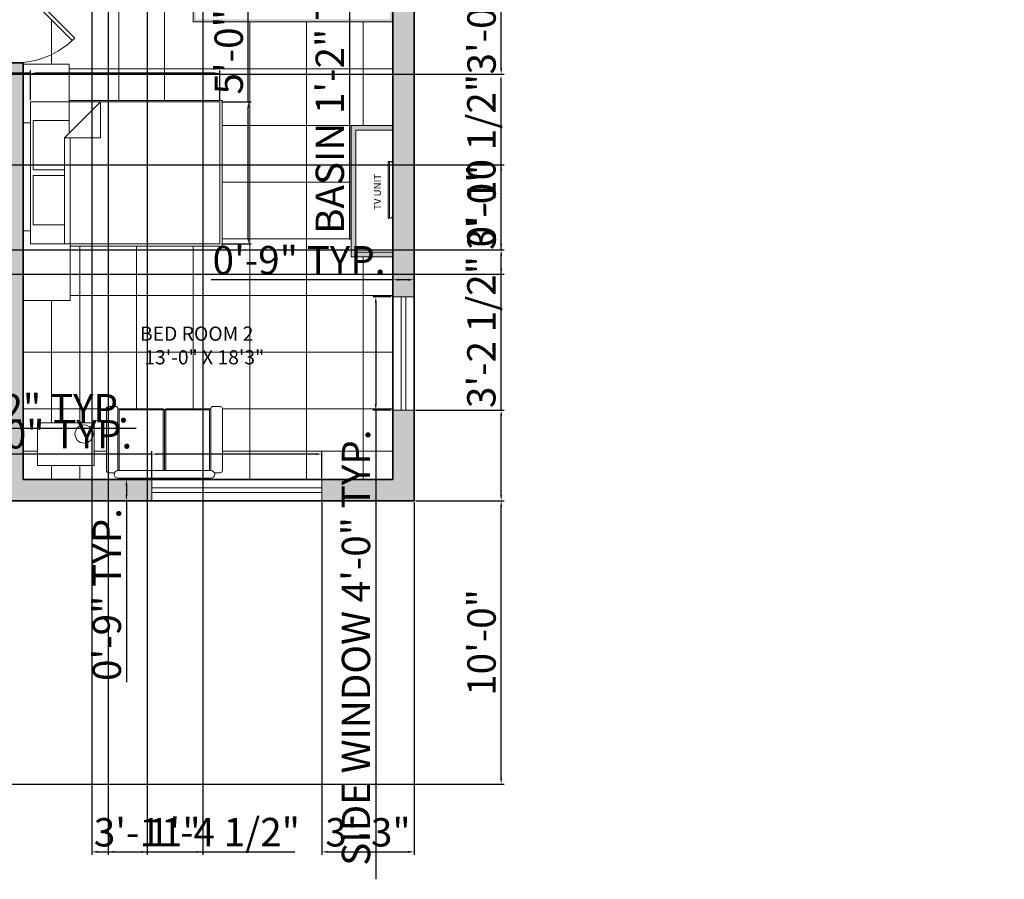
# Model space of a CAD drawing. Units: millimetres. Extents: x 542930 to 543750, y 628093 to 628738.
# Tile 8 of 14: x 543333 to 543750, y 628093 to 628458. Entities that reach past the tile are written whole.
import ezdxf

# ---------------------------------------------------------------- set-up
doc = ezdxf.new("R2010")
doc.units = ezdxf.units.MM
for name, color, linetype, lineweight in [('A-ANNO-DIMS', 2, 'Continuous', 18), ('A-EQPM', 9, 'Continuous', 18), ('A-EQPM-PATT', 9, 'Continuous', 13), ('A-FURN', 8, 'Continuous', 18), ('A-FURN-MILL', 8, 'Continuous', 18), ('A-FURN-PATT', 9, 'Continuous', 13), ('A-WALL', 7, 'Continuous', 35), ('DOORS', 30, 'Continuous', 18), ('WINDOW', 70, 'Continuous', 18)]:
    doc.layers.add(name, color=color, linetype=linetype, lineweight=lineweight)
for name, color, linetype, lineweight, true_color in [('A-ANNO-TEXT', 40, 'Continuous', 18, 0xf8d731), ('A-AREA-IDEN', 40, 'Continuous', 18, 0xf8d731), ('A-FLOR-PATT', 241, 'Continuous', 13, 0xf7abae), ('A-WALL-PATT', 251, 'Continuous', 13, 0x636466)]:
    doc.layers.add(name, color=color, linetype=linetype, lineweight=lineweight, true_color=true_color)
doc.styles.get("Standard").update_dxf_attribs({"font": 'arial.ttf'})
doc.dimstyles.new('ISO-25', dxfattribs={"dimtxt": 12, "dimasz": 2.5, "dimexe": 1.25, "dimexo": 0.625, "dimtad": 1, "dimdec": 0, "dimlunit": 3, "dimtxsty": 'Standard', "dimcen": 2.5, "dimadec": 0, "dimazin": 0, "dimtfac": 1, "dimtdec": 0, "dimtmove": 0, "dimatfit": 3, "dimfxl": 1, "dimarcsym": 0})

# ---------------------------------------------------------------- blocks, each defined once
blk = doc.blocks.new('*U2')
for p, q in [((0, 0), (0, -6)), ((40, 0), (40, -6))]:
    blk.add_line(p, q)
blk.add_lwpolyline([(0, 0), (28.28, 28.28), (29.52, 27.05), (1.24, -1.24)], close=True)
blk.add_arc((0, 0), 40, 0, 45)
blk = doc.blocks.new('Bed - Queen')
for p, q in [((0, -80.00003), (0, 0)), ((0, 0), (59.99999, 0)), ((59.99999, 0), (59.99999, -80.00003)), ((7.99999, -1.2), (28.79998, -1.2)), ((7.99999, -14.4), (7.99999, -1.2)), ((28.79998, -1.2), (28.79998, -14.4)), ((31.19999, -1.2), (51.99999, -1.2)), ((31.19999, -14.4), (31.19999, -1.2)), ((51.99999, -1.2), (51.99999, -16.4)), ((0, -14.4), (44.8, -14.4)), ((59.99999, -29.6), (44.8, -14.4)), ((44.8, -14.4), (44.8, -29.6)), ((51.99999, -16.4), (46.79936, -16.4)), ((44.8, -16.8), (0, -16.8)), ((44.8, -29.6), (59.99999, -29.6)), ((59.99999, -80.00003), (0, -80.00003))]:
    blk.add_line(p, q)
blk = doc.blocks.new('sofa')
for p, q in [((543001.62, 628230.38), (543001.62, 628182.38)), ((543010.62, 628230.38), (543045.62, 628230.38)), ((543091.62, 628230.38), (543091.62, 628182.38)), ((543045.62, 628229.38), (543045.62, 628182.38)), ((543046.62, 628228.78), (543046.62, 628182.38)), ((543010.62, 628176.38), (543082.62, 628176.38))]:
    blk.add_line(p, q)
for points in [[(543009.53, 628232.06), (543003.46, 628232.06, 0.414214), (543001.62, 628230.23)], [(543045.62, 628230.38, 0.623864), (543047.62, 628230.38), (543082.62, 628230.38), (543082.62, 628182.38), (543010.62, 628182.38), (543010.62, 628230.38, 0.297291), (543009.53, 628232.06)], [(543083.72, 628232.06, 0.297291), (543082.62, 628230.38), (543082.62, 628182.38)], [(543091.62, 628230.23, 0.414214), (543089.79, 628232.06), (543083.72, 628232.06)], [(543001.62, 628182.54, 0.414214), (543003.46, 628180.7), (543007.93, 628180.7)], [(543082.62, 628182.38, -1), (543082.62, 628176.38), (543082.62, 628175.38), (543010.62, 628175.38), (543010.62, 628176.38, -1), (543010.62, 628182.38)], [(543085.32, 628180.7), (543089.79, 628180.7, 0.414214), (543091.62, 628182.54)]]:
    blk.add_lwpolyline(points, format="xyb")
for points in [[(543011.62, 628182.38), (543011.62, 628229.38), (543045.62, 628229.38), (543045.62, 628229.4)], [(543047.62, 628182.38), (543047.62, 628229.38), (543047.62, 628229.4)], [(543047.62, 628229.38), (543081.62, 628229.38), (543081.62, 628182.38)]]:
    blk.add_lwpolyline(points)
blk.add_arc((543046.62, 628229.89), 1.11, 206.0829, 333.9171)
blk = doc.blocks.new('BEDROOM-END-TABLE')
for p, q in [((0, 0), (0, 18)), ((24.02, 18), (0, 18)), ((24.02, 0), (24.02, 18)), ((24.02, 0), (0, 0))]:
    blk.add_line(p, q)
blk.add_circle((19.74, 13.28), 3.85)
blk = doc.blocks.new('WIN-BEDROOM-FRONT')
for p, q in [((0, 9), (0, 0)), ((72, 9), (72, 0)), ((0, 5.5), (72, 5.5)), ((0, 3.5), (72, 3.5))]:
    blk.add_line(p, q)
blk = doc.blocks.new('WIN-BEDROOM-SIDE')
for p, q in [((0, 48), (9, 48)), ((3.5, 48), (3.5, 0)), ((5.5, 48), (5.5, 0)), ((0, 0), (9, 0))]:
    blk.add_line(p, q)
blk = doc.blocks.new('BED-SIDE-STAND')
for p, q in [((19.46, 24), (0, 24)), ((19.46, 0), (19.46, 24))]:
    blk.add_line(p, q)
blk = doc.blocks.new('*D35')
at = {"layer": 'A-ANNO-DIMS', "color": 0, "lineweight": -2, "transparency": 16777216}
for p, q in [((543473.87, 628509.97), (543471.13, 628509.97)), ((543472.38, 628507.47), (543472.38, 628498.35)), ((543473.87, 628495.85), (543471.13, 628495.85)), ((543472.38, 628495.85), (543472.38, 628364.52))]:
    blk.add_line(p, q, dxfattribs=at)
at = {"layer": 'A-ANNO-DIMS', "color": 0, "transparency": 16777216}
for points in [[(543471.96, 628507.47), (543472.79, 628507.47), (543472.38, 628509.97)], [(543471.96, 628498.35), (543472.79, 628498.35), (543472.38, 628495.85)]]:
    blk.add_solid(points, dxfattribs=at)
at = {"layer": 'Defpoints', "color": 0, "transparency": 16777216}
for p in [(543474.49, 628509.97), (543472.38, 628495.85), (543474.49, 628495.85)]:
    blk.add_point(p, dxfattribs=at)
at = {"layer": 'A-ANNO-DIMS', "color": 0, "transparency": 16777216, "insert": (543465.55, 628428.93), "char_height": 12, "attachment_point": 5, "rotation": 90}
blk.add_mtext('BASIN 1\'-2" TYP.', dxfattribs=at)
blk = doc.blocks.new('*D37')
at = {"layer": 'A-ANNO-DIMS', "color": 0, "lineweight": -2, "transparency": 16777216}
for p, q in [((543337.17, 628434.96), (543128.93, 628434.96)), ((543337.17, 628423.55), (543337.17, 628436.21)), ((543414.94, 628434.96), (543339.67, 628434.96)), ((543417.44, 628423.55), (543417.44, 628436.21))]:
    blk.add_line(p, q, dxfattribs=at)
at = {"layer": 'A-ANNO-DIMS', "color": 0, "transparency": 16777216}
for points in [[(543339.67, 628435.38), (543339.67, 628434.55), (543337.17, 628434.96)], [(543414.94, 628435.38), (543414.94, 628434.55), (543417.44, 628434.96)]]:
    blk.add_solid(points, dxfattribs=at)
at = {"layer": 'Defpoints', "color": 0, "transparency": 16777216}
for p in [(543337.17, 628434.96), (543337.17, 628422.92), (543417.44, 628422.92)]:
    blk.add_point(p, dxfattribs=at)
at = {"layer": 'A-ANNO-DIMS', "color": 0, "transparency": 16777216, "insert": (543231.8, 628442.16), "char_height": 12, "attachment_point": 5}
blk.add_mtext('QUEEN BED 6\'-8 1/2" TYP.', dxfattribs=at)
blk = doc.blocks.new('*D38')
at = {"layer": 'A-ANNO-DIMS', "color": 0, "lineweight": -2, "transparency": 16777216}
for p, q in [((543429.48, 628422.92), (543429.48, 628499.82)), ((543418.07, 628422.92), (543430.73, 628422.92)), ((543429.48, 628365.22), (543429.48, 628420.42)), ((543418.07, 628362.72), (543430.73, 628362.72))]:
    blk.add_line(p, q, dxfattribs=at)
at = {"layer": 'A-ANNO-DIMS', "color": 0, "transparency": 16777216}
for points in [[(543429.07, 628420.42), (543429.9, 628420.42), (543429.48, 628422.92)], [(543429.07, 628365.22), (543429.9, 628365.22), (543429.48, 628362.72)]]:
    blk.add_solid(points, dxfattribs=at)
at = {"layer": 'Defpoints', "color": 0, "transparency": 16777216}
for p in [(543417.44, 628422.92), (543429.48, 628422.92), (543417.44, 628362.72)]:
    blk.add_point(p, dxfattribs=at)
at = {"layer": 'A-ANNO-DIMS', "color": 0, "transparency": 16777216, "insert": (543422.73, 628462.62), "char_height": 12, "attachment_point": 5, "rotation": 90}
blk.add_mtext('5\'-0" TYP.', dxfattribs=at)
blk = doc.blocks.new('*D41')
at = {"layer": 'A-ANNO-DIMS', "color": 0, "lineweight": -2, "transparency": 16777216}
for p, q in [((543177.94, 628290.42), (543177.94, 628283.41)), ((543220.5, 628290.42), (543220.5, 628283.41)), ((543180.44, 628284.66), (543218, 628284.66)), ((543220.5, 628284.66), (543382.04, 628284.66))]:
    blk.add_line(p, q, dxfattribs=at)
at = {"layer": 'A-ANNO-DIMS', "color": 0, "transparency": 16777216}
for points in [[(543180.44, 628285.08), (543180.44, 628284.25), (543177.94, 628284.66)], [(543218, 628285.08), (543218, 628284.25), (543220.5, 628284.66)]]:
    blk.add_solid(points, dxfattribs=at)
at = {"layer": 'Defpoints', "color": 0, "transparency": 16777216}
for p in [(543177.94, 628291.05), (543220.5, 628291.05), (543220.5, 628284.66)]:
    blk.add_point(p, dxfattribs=at)
at = {"layer": 'A-ANNO-DIMS', "color": 0, "transparency": 16777216, "insert": (543302.52, 628291.5), "char_height": 12, "attachment_point": 5}
blk.add_mtext('CHAIR 3\'-6 1/2" TYP.', dxfattribs=at)
blk = doc.blocks.new('*D45')
at = {"layer": 'A-ANNO-DIMS', "color": 0, "lineweight": -2, "transparency": 16777216}
for p, q in [((543407.17, 628481.45), (543407.17, 628494.45)), ((543409.67, 628493.2), (543487.17, 628493.2)), ((543489.67, 628481.45), (543489.67, 628494.45)), ((543489.67, 628493.2), (543749.65, 628493.2))]:
    blk.add_line(p, q, dxfattribs=at)
at = {"layer": 'A-ANNO-DIMS', "color": 0, "transparency": 16777216}
for points in [[(543409.67, 628493.62), (543409.67, 628492.78), (543407.17, 628493.2)], [(543487.17, 628493.62), (543487.17, 628492.78), (543489.67, 628493.2)]]:
    blk.add_solid(points, dxfattribs=at)
at = {"layer": 'Defpoints', "color": 0, "transparency": 16777216}
for p in [(543489.67, 628493.2), (543407.17, 628480.83), (543489.67, 628480.83)]:
    blk.add_point(p, dxfattribs=at)
at = {"layer": 'A-ANNO-DIMS', "color": 0, "transparency": 16777216, "insert": (543620.91, 628500.03), "char_height": 12, "attachment_point": 5}
blk.add_mtext('WARDROBE RAIL 6\'-10 1/2" TYP.', dxfattribs=at)
blk = doc.blocks.new('*D49')
at = {"layer": 'A-ANNO-DIMS', "color": 0, "lineweight": -2, "transparency": 16777216}
for p, q in [((543388.65, 628263.45), (543388.65, 628274.88)), ((543460.65, 628263.45), (543460.65, 628274.88)), ((543388.65, 628273.63), (543171.83, 628273.63)), ((543458.15, 628273.63), (543391.15, 628273.63))]:
    blk.add_line(p, q, dxfattribs=at)
at = {"layer": 'A-ANNO-DIMS', "color": 0, "transparency": 16777216}
for points in [[(543391.15, 628274.04), (543391.15, 628273.21), (543388.65, 628273.63)], [(543458.15, 628274.04), (543458.15, 628273.21), (543460.65, 628273.63)]]:
    blk.add_solid(points, dxfattribs=at)
at = {"layer": 'Defpoints', "color": 0, "transparency": 16777216}
for p in [(543388.65, 628273.63), (543388.65, 628262.83), (543460.65, 628262.83)]:
    blk.add_point(p, dxfattribs=at)
at = {"layer": 'A-ANNO-DIMS', "color": 0, "transparency": 16777216, "insert": (543278.99, 628280.46), "char_height": 12, "attachment_point": 5}
blk.add_mtext('FRONT WINDOW 6\'-0" TYP.', dxfattribs=at)
blk = doc.blocks.new('*D50')
at = {"layer": 'A-ANNO-DIMS', "color": 0, "lineweight": -2, "transparency": 16777216}
for p, q in [((543388.02, 628262.83), (543376.6, 628262.83)), ((543377.85, 628260.33), (543377.85, 628256.33)), ((543388.02, 628253.83), (543376.6, 628253.83)), ((543377.85, 628253.83), (543377.85, 628176.93))]:
    blk.add_line(p, q, dxfattribs=at)
at = {"layer": 'A-ANNO-DIMS', "color": 0, "transparency": 16777216}
for points in [[(543377.43, 628260.33), (543378.26, 628260.33), (543377.85, 628262.83)], [(543377.43, 628256.33), (543378.26, 628256.33), (543377.85, 628253.83)]]:
    blk.add_solid(points, dxfattribs=at)
at = {"layer": 'Defpoints', "color": 0, "transparency": 16777216}
for p in [(543388.65, 628262.83), (543377.85, 628253.83), (543388.65, 628253.83)]:
    blk.add_point(p, dxfattribs=at)
at = {"layer": 'A-ANNO-DIMS', "color": 0, "transparency": 16777216, "insert": (543371.09, 628214.13), "char_height": 12, "attachment_point": 5, "rotation": 90}
blk.add_mtext('0\'-9" TYP.', dxfattribs=at)
blk = doc.blocks.new('*D51')
at = {"layer": 'A-ANNO-DIMS', "color": 0, "lineweight": -2, "transparency": 16777216}
for p, q in [((543490.04, 628340.3), (543482.22, 628340.3)), ((543483.47, 628337.8), (543483.47, 628294.8)), ((543490.04, 628292.3), (543482.22, 628292.3)), ((543483.47, 628292.3), (543483.47, 628093.46))]:
    blk.add_line(p, q, dxfattribs=at)
at = {"layer": 'A-ANNO-DIMS', "color": 0, "transparency": 16777216}
for points in [[(543483.05, 628337.8), (543483.88, 628337.8), (543483.47, 628340.3)], [(543483.05, 628294.8), (543483.88, 628294.8), (543483.47, 628292.3)]]:
    blk.add_solid(points, dxfattribs=at)
at = {"layer": 'Defpoints', "color": 0, "transparency": 16777216}
for p in [(543490.67, 628340.3), (543483.47, 628292.3), (543490.67, 628292.3)]:
    blk.add_point(p, dxfattribs=at)
at = {"layer": 'A-ANNO-DIMS', "color": 0, "transparency": 16777216, "insert": (543476.63, 628191.63), "char_height": 12, "attachment_point": 5, "rotation": 90}
blk.add_mtext('SIDE WINDOW 4\'-0" TYP.', dxfattribs=at)
blk = doc.blocks.new('*D52')
at = {"layer": 'A-ANNO-DIMS', "color": 0, "lineweight": -2, "transparency": 16777216}
for p, q in [((543490.67, 628347.5), (543413.77, 628347.5)), ((543490.67, 628340.93), (543490.67, 628348.75)), ((543497.17, 628347.5), (543493.17, 628347.5)), ((543499.67, 628340.93), (543499.67, 628348.75))]:
    blk.add_line(p, q, dxfattribs=at)
at = {"layer": 'A-ANNO-DIMS', "color": 0, "transparency": 16777216}
for points in [[(543493.17, 628347.92), (543493.17, 628347.08), (543490.67, 628347.5)], [(543497.17, 628347.92), (543497.17, 628347.08), (543499.67, 628347.5)]]:
    blk.add_solid(points, dxfattribs=at)
at = {"layer": 'Defpoints', "color": 0, "transparency": 16777216}
for p in [(543490.67, 628347.5), (543490.67, 628340.3), (543499.67, 628340.3)]:
    blk.add_point(p, dxfattribs=at)
at = {"layer": 'A-ANNO-DIMS', "color": 0, "transparency": 16777216, "insert": (543450.97, 628354.25), "char_height": 12, "attachment_point": 5}
blk.add_mtext('0\'-9" TYP.', dxfattribs=at)
blk = doc.blocks.new('*D61')
at = {"layer": 'A-ANNO-DIMS', "color": 0, "lineweight": -2, "transparency": 16777216}
for p, q in [((543500.29, 628253.83), (543537.81, 628253.83)), ((543536.56, 628136.33), (543536.56, 628251.33)), ((543325.79, 628133.83), (543537.81, 628133.83))]:
    blk.add_line(p, q, dxfattribs=at)
at = {"layer": 'A-ANNO-DIMS', "color": 0, "transparency": 16777216}
for points in [[(543536.15, 628251.33), (543536.98, 628251.33), (543536.56, 628253.83)], [(543536.15, 628136.33), (543536.98, 628136.33), (543536.56, 628133.83)]]:
    blk.add_solid(points, dxfattribs=at)
at = {"layer": 'Defpoints', "color": 0, "transparency": 16777216}
for p in [(543499.67, 628253.83), (543536.56, 628253.83), (543325.17, 628133.83)]:
    blk.add_point(p, dxfattribs=at)
at = {"layer": 'A-ANNO-DIMS', "color": 0, "transparency": 16777216, "insert": (543529.81, 628193.83), "char_height": 12, "attachment_point": 5, "rotation": 90}
blk.add_mtext('10\'-0"', dxfattribs=at)
blk = doc.blocks.new('*D63')
at = {"layer": 'A-ANNO-DIMS', "color": 0, "lineweight": -2, "transparency": 16777216}
for p, q in [((543460.65, 628253.2), (543460.65, 628103.84)), ((543499.67, 628253.2), (543499.67, 628103.84)), ((543463.15, 628105.09), (543497.17, 628105.09))]:
    blk.add_line(p, q, dxfattribs=at)
at = {"layer": 'A-ANNO-DIMS', "color": 0, "transparency": 16777216}
for points in [[(543463.15, 628105.5), (543463.15, 628104.67), (543460.65, 628105.09)], [(543497.17, 628105.5), (543497.17, 628104.67), (543499.67, 628105.09)]]:
    blk.add_solid(points, dxfattribs=at)
at = {"layer": 'Defpoints', "color": 0, "transparency": 16777216}
for p in [(543460.65, 628253.83), (543499.67, 628253.83), (543499.67, 628105.09)]:
    blk.add_point(p, dxfattribs=at)
at = {"layer": 'A-ANNO-DIMS', "color": 0, "transparency": 16777216, "insert": (543480.16, 628111.84), "char_height": 12, "attachment_point": 5}
blk.add_mtext('3\'-3"', dxfattribs=at)
blk = doc.blocks.new('*D65')
at = {"layer": 'A-ANNO-DIMS', "color": 0, "lineweight": -2, "transparency": 16777216}
for p, q in [((543536.56, 628292.3), (543536.56, 628355.9)), ((543500.29, 628292.3), (543537.81, 628292.3)), ((543536.56, 628256.33), (543536.56, 628289.8)), ((543500.29, 628253.83), (543537.81, 628253.83))]:
    blk.add_line(p, q, dxfattribs=at)
at = {"layer": 'A-ANNO-DIMS', "color": 0, "transparency": 16777216}
for points in [[(543536.15, 628289.8), (543536.98, 628289.8), (543536.56, 628292.3)], [(543536.15, 628256.33), (543536.98, 628256.33), (543536.56, 628253.83)]]:
    blk.add_solid(points, dxfattribs=at)
at = {"layer": 'Defpoints', "color": 0, "transparency": 16777216}
for p in [(543499.67, 628292.3), (543536.56, 628292.3), (543499.67, 628253.83)]:
    blk.add_point(p, dxfattribs=at)
at = {"layer": 'A-ANNO-DIMS', "color": 0, "transparency": 16777216, "insert": (543529.73, 628325.35), "char_height": 12, "attachment_point": 5, "rotation": 90}
blk.add_mtext('3\'-2 1/2"', dxfattribs=at)
blk = doc.blocks.new('*D73')
at = {"layer": 'A-ANNO-DIMS', "color": 0, "lineweight": -2, "transparency": 16777216}
for p, q in [((543158.79, 628396.23), (543537.81, 628396.23)), ((543536.56, 628362.73), (543536.56, 628393.73)), ((543158.79, 628360.23), (543537.81, 628360.23))]:
    blk.add_line(p, q, dxfattribs=at)
at = {"layer": 'A-ANNO-DIMS', "color": 0, "transparency": 16777216}
for points in [[(543536.15, 628393.73), (543536.98, 628393.73), (543536.56, 628396.23)], [(543536.15, 628362.73), (543536.98, 628362.73), (543536.56, 628360.23)]]:
    blk.add_solid(points, dxfattribs=at)
at = {"layer": 'Defpoints', "color": 0, "transparency": 16777216}
for p in [(543158.17, 628396.23), (543536.56, 628396.23), (543158.17, 628360.23)]:
    blk.add_point(p, dxfattribs=at)
at = {"layer": 'A-ANNO-DIMS', "color": 0, "transparency": 16777216, "insert": (543529.81, 628378.23), "char_height": 12, "attachment_point": 5, "rotation": 90}
blk.add_mtext('3\'-0"', dxfattribs=at)
blk = doc.blocks.new('*D74')
at = {"layer": 'A-ANNO-DIMS', "color": 0, "lineweight": -2, "transparency": 16777216}
for p, q in [((543536.56, 628360.23), (543536.56, 628433.16)), ((543158.79, 628360.23), (543537.81, 628360.23)), ((543536.56, 628352.33), (543536.56, 628357.73)), ((543158.79, 628349.83), (543537.81, 628349.83))]:
    blk.add_line(p, q, dxfattribs=at)
at = {"layer": 'A-ANNO-DIMS', "color": 0, "transparency": 16777216}
for points in [[(543536.15, 628357.73), (543536.98, 628357.73), (543536.56, 628360.23)], [(543536.15, 628352.33), (543536.98, 628352.33), (543536.56, 628349.83)]]:
    blk.add_solid(points, dxfattribs=at)
at = {"layer": 'Defpoints', "color": 0, "transparency": 16777216}
for p in [(543158.17, 628360.23), (543536.56, 628360.23), (543158.17, 628349.83)]:
    blk.add_point(p, dxfattribs=at)
at = {"layer": 'A-ANNO-DIMS', "color": 0, "transparency": 16777216, "insert": (543529.73, 628397.95), "char_height": 12, "attachment_point": 5, "rotation": 90}
blk.add_mtext('0\'-10 1/2"', dxfattribs=at)
blk = doc.blocks.new('*D78')
at = {"layer": 'A-ANNO-DIMS', "color": 0, "lineweight": -2, "transparency": 16777216}
for p, q in [((543304.67, 628350.45), (543304.67, 628619.78)), ((543307.17, 628618.53), (543322.67, 628618.53)), ((543325.17, 628350.45), (543325.17, 628619.78)), ((543325.17, 628618.53), (543387.65, 628618.53))]:
    blk.add_line(p, q, dxfattribs=at)
at = {"layer": 'A-ANNO-DIMS', "color": 0, "transparency": 16777216}
for points in [[(543307.17, 628618.94), (543307.17, 628618.11), (543304.67, 628618.53)], [(543322.67, 628618.94), (543322.67, 628618.11), (543325.17, 628618.53)]]:
    blk.add_solid(points, dxfattribs=at)
at = {"layer": 'Defpoints', "color": 0, "transparency": 16777216}
for p in [(543325.17, 628618.53), (543304.67, 628349.83), (543325.17, 628349.83)]:
    blk.add_point(p, dxfattribs=at)
at = {"layer": 'A-ANNO-DIMS', "color": 0, "transparency": 16777216, "insert": (543357.66, 628625.36), "char_height": 12, "attachment_point": 5}
blk.add_mtext('1\'-8 1/2"', dxfattribs=at)
blk = doc.blocks.new('*D80')
at = {"layer": 'A-ANNO-DIMS', "color": 0, "lineweight": -2, "transparency": 16777216}
for p, q in [((543228.79, 628470.52), (543537.81, 628470.52)), ((543536.56, 628437.09), (543536.56, 628468.02)), ((543228.79, 628434.59), (543537.81, 628434.59))]:
    blk.add_line(p, q, dxfattribs=at)
at = {"layer": 'A-ANNO-DIMS', "color": 0, "transparency": 16777216}
for points in [[(543536.15, 628468.02), (543536.98, 628468.02), (543536.56, 628470.52)], [(543536.15, 628437.09), (543536.98, 628437.09), (543536.56, 628434.59)]]:
    blk.add_solid(points, dxfattribs=at)
at = {"layer": 'Defpoints', "color": 0, "transparency": 16777216}
for p in [(543228.16, 628470.52), (543536.56, 628470.52), (543228.16, 628434.59)]:
    blk.add_point(p, dxfattribs=at)
at = {"layer": 'A-ANNO-DIMS', "color": 0, "transparency": 16777216, "insert": (543529.81, 628452.55), "char_height": 12, "attachment_point": 5, "rotation": 90}
blk.add_mtext('3\'-0"', dxfattribs=at)
blk = doc.blocks.new('*D82')
at = {"layer": 'A-ANNO-DIMS', "color": 0, "lineweight": -2, "transparency": 16777216}
for p, q in [((543363.17, 628557.2), (543363.17, 628103.84)), ((543410.17, 628556.2), (543410.17, 628103.84)), ((543365.67, 628105.09), (543407.67, 628105.09))]:
    blk.add_line(p, q, dxfattribs=at)
at = {"layer": 'A-ANNO-DIMS', "color": 0, "transparency": 16777216}
for points in [[(543365.67, 628105.5), (543365.67, 628104.67), (543363.17, 628105.09)], [(543407.67, 628105.5), (543407.67, 628104.67), (543410.17, 628105.09)]]:
    blk.add_solid(points, dxfattribs=at)
at = {"layer": 'Defpoints', "color": 0, "transparency": 16777216}
for p in [(543363.17, 628557.83), (543410.17, 628556.83), (543410.17, 628105.09)]:
    blk.add_point(p, dxfattribs=at)
at = {"layer": 'A-ANNO-DIMS', "color": 0, "transparency": 16777216, "insert": (543386.67, 628111.84), "char_height": 12, "attachment_point": 5}
blk.add_mtext('3\'-11"', dxfattribs=at)
blk = doc.blocks.new('*D84')
at = {"layer": 'A-ANNO-DIMS', "color": 0, "lineweight": -2, "transparency": 16777216}
for p, q in [((543386.67, 628556.2), (543386.67, 628103.84)), ((543370.17, 628490.2), (543370.17, 628103.84)), ((543372.67, 628105.09), (543384.17, 628105.09)), ((543386.67, 628105.09), (543449.15, 628105.09))]:
    blk.add_line(p, q, dxfattribs=at)
at = {"layer": 'A-ANNO-DIMS', "color": 0, "transparency": 16777216}
for points in [[(543372.67, 628105.5), (543372.67, 628104.67), (543370.17, 628105.09)], [(543384.17, 628105.5), (543384.17, 628104.67), (543386.67, 628105.09)]]:
    blk.add_solid(points, dxfattribs=at)
at = {"layer": 'Defpoints', "color": 0, "transparency": 16777216}
for p in [(543386.67, 628556.83), (543370.17, 628490.83), (543386.67, 628105.09)]:
    blk.add_point(p, dxfattribs=at)
at = {"layer": 'A-ANNO-DIMS', "color": 0, "transparency": 16777216, "insert": (543419.16, 628111.92), "char_height": 12, "attachment_point": 5}
blk.add_mtext('1\'-4 1/2"', dxfattribs=at)

msp = doc.modelspace()

# ---------------------------------------------------------------- hatches: boundary and pattern name
at = {"layer": 'A-EQPM-PATT'}
h = msp.add_hatch(color=256, dxfattribs=at)
h.dxf.hatch_style = 1
h.paths.add_polyline_path([(543489.33, 628397.59), (543488.67, 628397.59), (543488.67, 628373.59), (543489.33, 628373.59)])
at = {"layer": 'A-FURN-PATT'}
h = msp.add_hatch(color=256, dxfattribs=at)
h.dxf.hatch_style = 1
h.paths.add_polyline_path([(543490.67, 628481.83), (543406.17, 628481.83), (543406.17, 628456.83), (543490.67, 628456.83)])
h.paths.add_polyline_path([(543407.17, 628480.83), (543489.67, 628480.83), (543489.67, 628457.83), (543407.17, 628457.83)], flags=16)
h.paths.add_polyline_path([(543409.15, 628477.78, -1), (543410.09, 628478.12), (543413.3, 628469.33), (543414.27, 628469.33), (543411.18, 628477.78, -1), (543412.12, 628478.12), (543415.34, 628469.33), (543416.03, 628469.33), (543412.94, 628477.78, -1), (543413.88, 628478.12), (543417.09, 628469.33), (543421.72, 628469.33), (543421.72, 628478.99, -1), (543422.72, 628478.99), (543422.72, 628469.33), (543427.97, 628469.33), (543431.33, 628478.53, -1), (543432.27, 628478.18), (543429.03, 628469.33), (543429.72, 628469.33), (543433.09, 628478.53, -1), (543434.03, 628478.18), (543430.79, 628469.33), (543431.55, 628469.33), (543434.91, 628478.53, -1), (543435.85, 628478.18), (543432.61, 628469.33), (543438.29, 628469.33), (543438.29, 628478.81, -1), (543439.29, 628478.81), (543439.29, 628469.33), (543440.2, 628469.33), (543440.2, 628478.81, -1), (543441.2, 628478.81), (543441.2, 628469.33), (543441.98, 628469.33), (543441.98, 628478.95, -1), (543442.98, 628478.95), (543442.98, 628469.33), (543443.68, 628469.33), (543443.68, 628479.02, -1), (543444.68, 628479.02), (543444.68, 628469.33), (543445.17, 628469.33), (543445.17, 628479.02, -1), (543446.17, 628479.02), (543446.17, 628469.33), (543451.08, 628469.33), (543454.37, 628478.31, -1), (543455.31, 628477.96), (543452.15, 628469.33), (543452.84, 628469.33), (543456.12, 628478.31, -1), (543457.06, 628477.96), (543453.9, 628469.33), (543454.88, 628469.33), (543458.16, 628478.31, -1), (543459.1, 628477.96), (543455.94, 628469.33), (543460.39, 628469.33), (543460.39, 628478.68, -1), (543461.39, 628478.68), (543461.39, 628469.33), (543462.17, 628469.33), (543462.17, 628478.56, -1), (543463.17, 628478.56), (543463.17, 628469.33), (543463.45, 628469.33), (543463.45, 628478.49, -1), (543464.45, 628478.49), (543464.45, 628469.33), (543465.03, 628469.33), (543465.03, 628478.49, -1), (543466.03, 628478.49), (543466.03, 628469.33), (543466.43, 628469.33), (543466.43, 628478.49, -1), (543467.43, 628478.49), (543467.43, 628469.33), (543471.19, 628469.33), (543474.18, 628477.48, -1), (543475.11, 628477.14), (543472.26, 628469.33), (543472.95, 628469.33), (543475.93, 628477.48, -1), (543476.87, 628477.14), (543474.01, 628469.33), (543478.55, 628469.33), (543481.53, 628477.48, -1), (543482.47, 628477.14), (543479.62, 628469.33), (543480.1, 628469.33), (543483.09, 628477.48, -1), (543484.02, 628477.14), (543477.84, 628460.23, -1), (543476.91, 628460.58), (543480.1, 628469.33), (543479.62, 628469.33), (543476.29, 628460.23, -1), (543475.35, 628460.58), (543478.55, 628469.33), (543474.01, 628469.33), (543470.69, 628460.23, -1), (543469.75, 628460.58), (543472.95, 628469.33), (543472.26, 628469.33), (543468.93, 628460.23, -1), (543468, 628460.58), (543471.19, 628469.33), (543467.43, 628469.33), (543467.43, 628460.49, -1), (543466.43, 628460.49), (543466.43, 628469.33), (543466.03, 628469.33), (543466.03, 628460.49, -1), (543465.03, 628460.49), (543465.03, 628469.33), (543464.45, 628469.33), (543464.45, 628460.49, -1), (543463.45, 628460.49), (543463.45, 628469.33), (543463.17, 628469.33), (543463.17, 628460.56, -1), (543462.17, 628460.56), (543462.17, 628469.33), (543461.39, 628469.33), (543461.39, 628460.68, -1), (543460.39, 628460.68), (543460.39, 628469.33), (543455.94, 628469.33), (543452.92, 628461.06, -1), (543451.98, 628461.4), (543454.88, 628469.33), (543453.9, 628469.33), (543450.88, 628461.06, -1), (543449.94, 628461.4), (543452.84, 628469.33), (543452.15, 628469.33), (543449.13, 628461.06, -1), (543448.19, 628461.4), (543451.08, 628469.33), (543446.17, 628469.33), (543446.17, 628461.02, -1), (543445.17, 628461.02), (543445.17, 628469.33), (543444.68, 628469.33), (543444.68, 628461.02, -1), (543443.68, 628461.02), (543443.68, 628469.33), (543442.98, 628469.33), (543442.98, 628460.95, -1), (543441.98, 628460.95), (543441.98, 628469.33), (543441.2, 628469.33), (543441.2, 628460.81, -1), (543440.2, 628460.81), (543440.2, 628469.33), (543439.29, 628469.33), (543439.29, 628460.81, -1), (543438.29, 628460.81), (543438.29, 628469.33), (543432.61, 628469.33), (543429.67, 628461.28, -1), (543428.73, 628461.62), (543431.55, 628469.33), (543430.79, 628469.33), (543427.85, 628461.28, -1), (543426.91, 628461.62), (543429.72, 628469.33), (543429.03, 628469.33), (543426.09, 628461.28, -1), (543425.15, 628461.62), (543427.97, 628469.33), (543422.72, 628469.33), (543422.72, 628460.99, -1), (543421.72, 628460.99), (543421.72, 628469.33), (543417.09, 628469.33), (543420.06, 628461.22, -1), (543419.12, 628460.87), (543416.03, 628469.33), (543415.34, 628469.33), (543418.3, 628461.22, -1), (543417.36, 628460.87), (543414.27, 628469.33), (543413.3, 628469.33), (543416.27, 628461.22, -1), (543415.33, 628460.87)], flags=0)
h = msp.add_hatch(color=256, dxfattribs=at)
h.dxf.hatch_style = 1
h.paths.add_polyline_path([(543475.06, 628410.83), (543490.67, 628410.83), (543490.67, 628412.83), (543473.06, 628412.83), (543473.06, 628357.14), (543490.67, 628357.14), (543490.67, 628359.14), (543475.06, 628359.14)])
at = {"layer": 'A-WALL-PATT'}
h = msp.add_hatch(color=256, dxfattribs=at)
h.dxf.hatch_style = 1
h.paths.add_polyline_path([(543499.67, 628589.83), (543478.53, 628589.83), (543478.53, 628580.83), (543490.67, 628580.83), (543490.67, 628490.83), (543414.67, 628490.83), (543414.67, 628494.86), (543410.17, 628494.86), (543410.17, 628490.83), (543406.17, 628490.83), (543406.17, 628481.83), (543490.67, 628481.83), (543490.67, 628340.3), (543499.67, 628340.3)])
h = msp.add_hatch(color=256, dxfattribs=at)
h.dxf.hatch_style = 1
h.paths.add_polyline_path([(543388.65, 628262.83), (543374.28, 628262.83), (543334.17, 628262.83), (543334.17, 628439.36), (543325.17, 628439.36), (543325.17, 628349.83), (543277.67, 628349.83), (543277.67, 628340.83), (543325.17, 628340.83), (543325.17, 628253.83), (543388.65, 628253.83)])
h = msp.add_hatch(color=256, dxfattribs=at)
h.dxf.hatch_style = 1
h.paths.add_polyline_path([(543499.67, 628292.3), (543490.67, 628292.3), (543490.67, 628262.83), (543460.65, 628262.83), (543460.65, 628253.83), (543499.67, 628253.83)])

# ---------------------------------------------------------------- linework, layer by layer
at = {"layer": 'A-EQPM'}
for p, q in [((543488.67, 628373.59), (543488.67, 628397.59)), ((543488.67, 628397.59), (543489.33, 628397.59)), ((543489.33, 628373.59), (543489.33, 628397.59)), ((543488.67, 628373.59), (543489.33, 628373.59))]:
    msp.add_line(p, q, dxfattribs=at)
for centre, start, end in [((543489.29, 628395.83), 38.3608, 88.5091), ((543489.29, 628375.34), 271.4909, 321.6392)]:
    msp.add_arc(centre, 1.76, start, end, dxfattribs=at)
at = {"layer": 'A-FLOR-PATT'}
for p, q in [((543374.7, 628423.51), (543374.7, 628556.83)), ((543393.93, 628423.51), (543393.93, 628547.28)), ((543346.17, 628438.89), (543346.17, 628457.54)), ((543430.17, 628262.83), (543430.17, 628456.83)), ((543454.17, 628262.83), (543454.17, 628456.83)), ((543478.17, 628412.83), (543478.17, 628456.83)), ((543353.62, 628436.83), (543490.67, 628436.83)), ((543418.47, 628412.83), (543473.06, 628412.83)), ((543418.47, 628388.83), (543473.06, 628388.83)), ((543418.47, 628364.83), (543473.06, 628364.83)), ((543358.17, 628286.83), (543358.17, 628361.72)), ((543382.17, 628292.83), (543382.17, 628361.72)), ((543406.17, 628292.83), (543406.17, 628361.72)), ((543478.17, 628262.83), (543478.17, 628357.14)), ((543346.17, 628286.83), (543346.17, 628338.72)), ((543354.02, 628340.83), (543490.67, 628340.83)), ((543334.17, 628316.83), (543490.67, 628316.83)), ((543334.17, 628292.83), (543369.37, 628292.83)), ((543418.51, 628292.83), (543490.67, 628292.83)), ((543334.17, 628274.83), (543340.17, 628274.83)), ((543364.19, 628274.83), (543369.37, 628274.83)), ((543418.51, 628274.83), (543490.67, 628274.83)), ((543346.17, 628262.83), (543346.17, 628268.83)), ((543358.17, 628262.83), (543358.17, 628268.83))]:
    msp.add_line(p, q, dxfattribs=at)
at = {"layer": 'A-FURN'}
for p, q in [((543353.62, 628423.51), (543418.47, 628423.51)), ((543418.47, 628423.51), (543418.47, 628361.72)), ((543337.17, 628413.97), (543334.17, 628413.97)), ((543337.17, 628368.25), (543334.17, 628368.25)), ((543354.02, 628362.72), (543354.02, 628338.72)), ((543418.47, 628361.72), (543354.02, 628361.72)), ((543354.02, 628338.72), (543334.17, 628338.72))]:
    msp.add_line(p, q, dxfattribs=at)
at = {"layer": 'A-FURN-MILL'}
for p, q in [((543406.17, 628490.83), (543406.17, 628456.83)), ((543406.17, 628456.83), (543490.67, 628456.83)), ((543473.06, 628412.83), (543473.06, 628357.14)), ((543473.06, 628412.83), (543490.67, 628412.83)), ((543475.06, 628410.83), (543475.06, 628359.14)), ((543475.06, 628410.83), (543490.67, 628410.83)), ((543475.06, 628359.14), (543490.67, 628359.14)), ((543473.06, 628357.14), (543490.67, 628357.14))]:
    msp.add_line(p, q, dxfattribs=at)
at = {"layer": 'A-WALL'}
for p, q in [((543499.67, 628589.83), (543499.67, 628253.83)), ((543490.67, 628481.83), (543490.67, 628262.83)), ((543334.17, 628439.36), (543325.17, 628439.36)), ((543334.17, 628262.83), (543334.17, 628439.36)), ((543388.65, 628262.83), (543334.17, 628262.83)), ((543388.65, 628262.83), (543490.67, 628262.83))]:
    msp.add_line(p, q, dxfattribs=at)
msp.add_lwpolyline([(543499.67, 628253.83), (542983.67, 628253.83), (542983.67, 628589.83)], dxfattribs=at)

# ---------------------------------------------------------------- block references
at = {"layer": 'A-FURN'}
for name, p in [('BED-SIDE-STAND', (543334.17, 628414.89)), ('BEDROOM-END-TABLE', (543340.17, 628268.83))]:
    msp.add_blockref(name, p, dxfattribs=at)
at = {"layer": 'A-FURN', "xscale": 1.003451310197957, "yscale": 1.003451310197957, "zscale": 1.003451310197957, "rotation": 90.00000000000003}
msp.add_blockref('Bed - Queen', (543337.17, 628362.72), dxfattribs=at)
at = {"layer": 'A-FURN', "xscale": 0.5460747824189197, "yscale": 0.5460747824189197, "zscale": 0.5460747824189197}
msp.add_blockref('sofa', (246849.87, 285232.09), dxfattribs=at)
at = {"layer": 'DOORS', "xscale": 0.8999999999970896, "yscale": 0.8999999999970896, "zscale": 0.8999999999970896, "rotation": 270}
msp.add_blockref('*U2', (543330.57, 628475.36), dxfattribs=at)
at = {"layer": 'WINDOW', "rotation": 180}
for name, p in [('WIN-BEDROOM-SIDE', (543499.67, 628340.3)), ('WIN-BEDROOM-FRONT', (543460.64, 628262.83))]:
    msp.add_blockref(name, p, dxfattribs=at)

# ---------------------------------------------------------------- texts
at = {"layer": 'A-ANNO-TEXT', "insert": (543482.66, 628375.25), "char_height": 3, "attachment_point": 1, "rotation": 90}
msp.add_mtext_dynamic_manual_height_columns('  TV UNIT', width=44.748, gutter_width=12.5, heights=[0], dxfattribs=at)
at = {"layer": 'A-AREA-IDEN', "insert": (543379.93, 628327.65), "char_height": 6, "attachment_point": 1}
msp.add_mtext_dynamic_manual_height_columns('  BED ROOM 2\\P   13\'-0" X 18\'3"', width=63.3037, gutter_width=12.5, heights=[0], dxfattribs=at)

# ---------------------------------------------------------------- dimensions: what is measured, and where the dimension line sits
at = {"layer": 'A-ANNO-DIMS'}
for base, p1, p2, picture, middle in [((543325.17, 628618.53), (543304.67, 628349.83), (543325.17, 628349.83), '*D78', (543357.66, 628625.36)), ((543410.17, 628105.09), (543363.17, 628557.83), (543410.17, 628556.83), '*D82', (543386.67, 628111.84)), ((543386.67, 628105.09), (543370.17, 628490.83), (543386.67, 628556.83), '*D84', (543419.16, 628111.92)), ((543499.67, 628105.09), (543460.65, 628253.83), (543499.67, 628253.83), '*D63', (543480.16, 628111.84))]:
    dim = msp.add_linear_dim(base=base, p1=p1, p2=p2, dimstyle='ISO-25', override={"dimdec": 1, "dimlfac": 1, "dimrnd": 0, "dimzin": 1, "dimdsep": 46, "dimlunit": 4, "dimfrac": 2}, dxfattribs=at)
    dim.commit()
    dim.dimension.update_dxf_attribs({"geometry": picture, "text_midpoint": middle})
for base, p1, p2, text, picture, middle in [((543489.67, 628493.2), (543407.17, 628480.83), (543489.67, 628480.83), 'WARDROBE RAIL <> TYP.', '*D45', (543620.91, 628500.03)), ((543220.5, 628284.66), (543177.94, 628291.05), (543220.5, 628291.05), 'CHAIR <> TYP.', '*D41', (543302.52, 628291.5))]:
    dim = msp.add_linear_dim(base=base, p1=p1, p2=p2, text=text, dimstyle='ISO-25', override={"dimdec": 1, "dimlfac": 1, "dimrnd": 0, "dimzin": 1, "dimdsep": 46, "dimlunit": 4, "dimfrac": 2}, dxfattribs=at)
    dim.commit()
    dim.dimension.update_dxf_attribs({"geometry": picture, "text_midpoint": middle})
for base, p1, p2, angle, text, picture, middle in [((543472.38, 628495.85), (543474.49, 628509.97), (543474.49, 628495.85), 270, 'BASIN <> TYP.', '*D35', (543465.55, 628428.93)), ((543429.48, 628422.92), (543417.44, 628362.72), (543417.44, 628422.92), 90, '<> TYP.', '*D38', (543422.73, 628462.62)), ((543337.17, 628434.96), (543417.44, 628422.92), (543337.17, 628422.92), 180, 'QUEEN BED <> TYP.', '*D37', (543231.8, 628442.16)), ((543490.67, 628347.5), (543499.67, 628340.3), (543490.67, 628340.3), 180, '<> TYP.', '*D52', (543450.97, 628354.25)), ((543483.47, 628292.3), (543490.67, 628340.3), (543490.67, 628292.3), 270, 'SIDE WINDOW <> TYP.', '*D51', (543476.63, 628191.63)), ((543388.65, 628273.63), (543460.65, 628262.83), (543388.65, 628262.83), 180, 'FRONT WINDOW <> TYP.', '*D49', (543278.99, 628280.46)), ((543377.85, 628253.83), (543388.65, 628262.83), (543388.65, 628253.83), 270, '<> TYP.', '*D50', (543371.09, 628214.13))]:
    dim = msp.add_linear_dim(base=base, p1=p1, p2=p2, angle=angle, text=text, dimstyle='ISO-25', override={"dimdec": 1, "dimlfac": 1, "dimrnd": 0, "dimzin": 1, "dimdsep": 46, "dimlunit": 4, "dimfrac": 2}, dxfattribs=at)
    dim.commit()
    dim.dimension.update_dxf_attribs({"geometry": picture, "text_midpoint": middle})
for base, p1, p2, picture, middle in [((543536.56, 628470.52), (543228.16, 628434.59), (543228.16, 628470.52), '*D80', (543529.81, 628452.55)), ((543536.56, 628360.23), (543158.17, 628349.83), (543158.17, 628360.23), '*D74', (543529.73, 628397.95)), ((543536.56, 628396.23), (543158.17, 628360.23), (543158.17, 628396.23), '*D73', (543529.81, 628378.23)), ((543536.56, 628292.3), (543499.67, 628253.83), (543499.67, 628292.3), '*D65', (543529.73, 628325.35)), ((543536.56, 628253.83), (543325.17, 628133.83), (543499.67, 628253.83), '*D61', (543529.81, 628193.83))]:
    dim = msp.add_linear_dim(base=base, p1=p1, p2=p2, angle=90, dimstyle='ISO-25', override={"dimdec": 1, "dimlfac": 1, "dimrnd": 0, "dimzin": 1, "dimdsep": 46, "dimlunit": 4, "dimfrac": 2}, dxfattribs=at)
    dim.commit()
    dim.dimension.update_dxf_attribs({"geometry": picture, "text_midpoint": middle})

doc.saveas('drawing.dxf')
